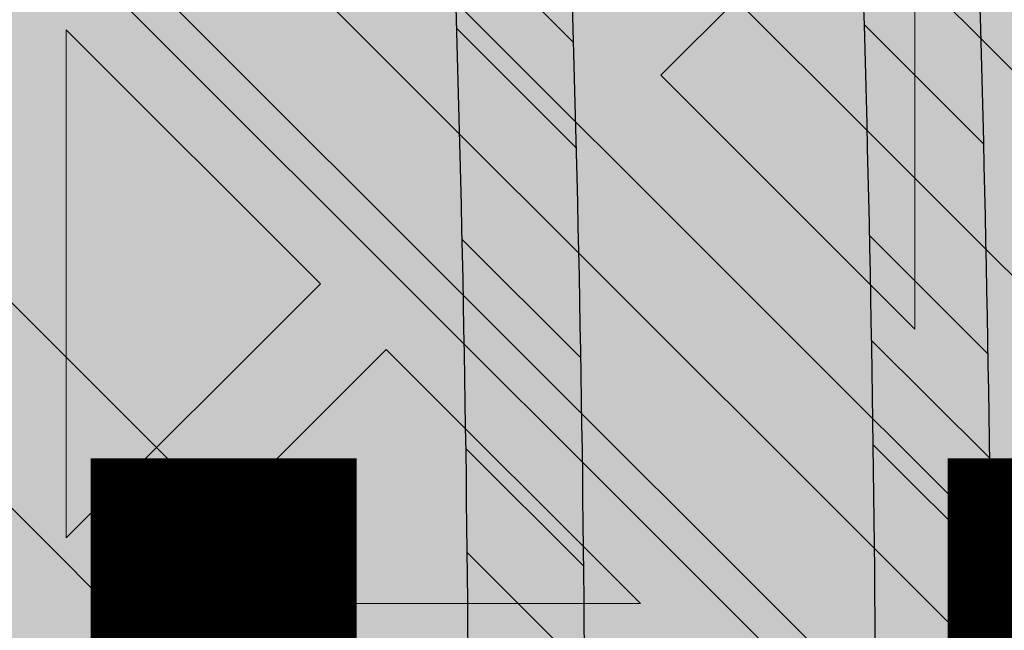
# Model space of a CAD drawing. Units: inches. Extents: x 844 to 2234, y 346 to 1084.
# Tile 80 of 93: x 2003.858 to 2006.557, y 703.938 to 705.614. Entities that reach past the tile are written whole.
import ezdxf

# ---------------------------------------------------------------- set-up
doc = ezdxf.new("R2010")
doc.units = ezdxf.units.IN
doc.header["$MEASUREMENT"] = 0
for name, color, linetype, lineweight in [('A-ANNO-DIMS', 2, 'Continuous', 18), ('furniture', 8, 'Continuous', 18), ('RA-AP-01$0$INT', 35, 'Continuous', 5)]:
    doc.layers.add(name, color=color, linetype=linetype, lineweight=lineweight)
doc.layers.add('RA-AP-01$0$FURN', color=3, linetype='Continuous')
doc.layers.add('RA-AP-01$0$WOOD', color=64, linetype='Continuous')
doc.styles.get("Standard").update_dxf_attribs({"font": 'arial.ttf'})
doc.dimstyles.get("Standard").update_dxf_attribs({"dimtxt": 6, "dimasz": 3, "dimexe": 0.18, "dimexo": 0.0625, "dimgap": 0.09, "dimtad": 0, "dimtih": 1, "dimtoh": 1, "dimdec": 1, "dimzin": 0, "dimdsep": 46, "dimlunit": 3, "dimtxsty": 'Standard', "dimblk": 'ARCHTICK', "dimcen": 0.09, "dimadec": 0, "dimazin": 0, "dimtfac": 1, "dimtdec": 1, "dimtofl": 0, "dimtmove": 0, "dimatfit": 3, "dimfxl": 1, "dimtolj": 1, "dimtzin": 0, "dimarcsym": 0})

# ---------------------------------------------------------------- blocks, each defined once
blk = doc.blocks.new('A$C18D01794')
at = {"layer": 'RA-AP-01$0$INT'}
h = blk.add_hatch(color=256, dxfattribs=at)
h.paths.add_polyline_path([(4.585917135068448, -7.856712009587804), (4.614201406330596, -7.856712009587056), (4.668846067270487, -7.802067348644738), (4.723490728212344, -7.856712009584164), (4.771774999457151, -7.856712009582887), (4.826419660396886, -7.80206734864072), (4.862780050090322, -7.838427738332541), (4.844495778842715, -7.856712009580965), (4.862780050090411, -7.856712009580482), (4.905206456960182, -7.814285602707865), (4.947632863832445, -7.856712009578238), (4.965917135079675, -7.856712009577755), (4.947632863831759, -7.838427738330656), (4.983993253523576, -7.802067348637219), (5.038637914464627, -7.856712009575829), (5.08692218571208, -7.856712009574554), (5.141566846649976, -7.802067348634224), (5.196211507589851, -7.856712009571666), (5.224495778822615, -7.856712009570916), (4.905206456953975, -7.537422687702283)])
h.paths.add_polyline_path([(4.895206456956031, -7.575706958950402), (4.895206456958921, -7.684996280828174), (4.840561796018589, -7.630351619890275)], flags=16)
h.paths.add_polyline_path([(4.915206456955638, -7.575706958949956), (4.969851117895509, -7.630351619887399), (4.915206456957609, -7.684996280827732)], flags=16)
h.paths.add_polyline_path([(4.826419660395175, -7.644493755514321), (4.881064321335613, -7.699138416452331), (4.771774999456703, -7.69913841645522)], flags=16)
h.paths.add_polyline_path([(4.983993253519558, -7.644493755510815), (5.038637914460456, -7.699138416449285), (4.929348592581548, -7.69913841645126)], flags=16)
h.paths.add_polyline_path([(4.881064321336025, -7.719138416452334), (4.826419660397532, -7.773783077393256), (4.771774999457062, -7.719138416455217)], flags=16)
h.paths.add_polyline_path([(4.929348592582019, -7.71913841645126), (5.038637914460982, -7.719138416449284), (4.983993253522945, -7.773783077389749)], flags=16)
h.paths.add_polyline_path([(4.895206456960191, -7.733280552075633), (4.895206456962115, -7.806001331460164), (4.876922185715016, -7.824285602708492), (4.840561796021581, -7.787925213016675)], flags=16)
h.paths.add_polyline_path([(4.915206456958487, -7.733280552075187), (4.969851117899527, -7.787925213013798), (4.933490728206909, -7.824285602708034), (4.9152064569598, -7.806001331461736)], flags=16)
h.paths.add_polyline_path([(4.757632863832376, -7.733280552079264), (4.812277524772842, -7.787925213017304), (4.757632863834348, -7.842569873958233)], flags=16)
h.paths.add_polyline_path([(4.737632863832376, -7.73328055207979), (4.737632863834348, -7.842569873958701), (4.682988202893906, -7.787925213020692)], flags=16)
h.paths.add_polyline_path([(5.05278005008503, -7.733280552072701), (5.052780050087917, -7.842569873951664), (4.998135389146995, -7.787925213013169)], flags=16)
h.paths.add_polyline_path([(5.072780050085024, -7.733280552072333), (5.127424711025931, -7.787925213010806), (5.072780050087916, -7.842569873951244)], flags=16)
h.paths.add_polyline_path([(4.935917135072783, -7.506712009583784), (5.255206456948811, -7.826001331459767), (5.255206456948932, -7.797717060211899), (5.200561796010279, -7.743072399273238), (5.255206456949403, -7.688427738334128), (5.25520645694961, -7.640143467086677), (5.200561796009787, -7.585498806146837), (5.236922185702417, -7.549138416454212), (5.255206456949919, -7.56742268770172), (5.255206456949998, -7.549138416454178), (5.212780050078687, -7.506712009583814), (5.25520645695036, -7.464285602712145), (5.255206456950438, -7.446001331464763), (5.236922185702424, -7.464285602712779), (5.200561796009796, -7.427925213020149), (5.255206456950753, -7.373280552079203), (5.25520645695096, -7.324996280834394), (5.200561796010322, -7.270351619893748), (5.255206456951428, -7.215706958952649), (5.255206456951547, -7.187422687705071)])
h.paths.add_polyline_path([(5.042988202883395, -7.42792521302065), (5.097632863823085, -7.373280552080975), (5.097632863822622, -7.482569873959883)], flags=16)
h.paths.add_polyline_path([(5.028846067259663, -7.442067348644384), (5.083490728198774, -7.496712009583504), (4.974201406321001, -7.496712009583035)], flags=16)
h.paths.add_polyline_path([(5.117632863823087, -7.37328055208089), (5.172277524762331, -7.42792521302015), (5.11763286382262, -7.482569873959851)], flags=16)
h.paths.add_polyline_path([(5.08349072819877, -7.516712009582191), (5.028846067259652, -7.571356670521302), (4.974201406320998, -7.516712009582638)], flags=16)
h.paths.add_polyline_path([(5.131774999446817, -7.35913841645716), (5.186419660386065, -7.413783077396415), (5.241064321325782, -7.359138416456712)], flags=17)
h.paths.add_polyline_path([(5.131774999446228, -7.496712009583703), (5.186419660386065, -7.442067348643883), (5.222780050079488, -7.478427738337313), (5.204495778832781, -7.496712009584014)], flags=16)
h.paths.add_polyline_path([(5.097632863822613, -7.530854145205813), (5.097632863823061, -7.640143467084723), (5.042988202883383, -7.585498806145032)], flags=16)
h.paths.add_polyline_path([(5.131774999446899, -7.339138416457162), (5.241064321325809, -7.339138416456712), (5.186419660386591, -7.284493755517479)], flags=17)
h.paths.add_polyline_path([(5.131774999446226, -7.516712009581999), (5.204495778830767, -7.516712009581702), (5.22278005007868, -7.534996280829206), (5.186419660386049, -7.571356670521828)], flags=16)
h.paths.add_polyline_path([(5.11763286382262, -7.530854145205852), (5.17227752476232, -7.585498806145562), (5.117632863823064, -7.64014346708481)], flags=16)
h.paths.add_polyline_path([(5.186419660386069, -7.599640941770585), (5.241064321325754, -7.654285602710281), (5.131774999446791, -7.654285602709814)], flags=16)
h.paths.add_polyline_path([(5.131774999446872, -7.674285602709813), (5.24106432132578, -7.674285602710282), (5.186419660386554, -7.728930263649504)], flags=16)
h.paths.add_polyline_path([(5.255206456951811, -7.126001331467467), (5.255206456951895, -7.106712009588038), (4.555206456956052, -7.106712009588038), (4.555206456956136, -7.12600133146746), (4.905206456953973, -7.476001331465289)])
h.paths.add_polyline_path([(4.983993253513404, -7.368930263651977), (4.92934859257295, -7.314285602713969), (5.03863791445186, -7.314285602711063)], flags=16)
h.paths.add_polyline_path([(4.969851117889988, -7.383072399276016), (4.915206456952556, -7.437717060215906), (4.915206456949648, -7.328427738338133)], flags=16)
h.paths.add_polyline_path([(4.929348592572535, -7.294285602713971), (4.983993253511019, -7.239640941773039), (5.038637914451496, -7.294285602711065)], flags=16)
h.paths.add_polyline_path([(5.052780050074912, -7.280143467087016), (4.998135389134438, -7.225498806148989), (5.052780050072919, -7.170854145208052)], flags=16)
h.paths.add_polyline_path([(5.07278005007491, -7.280143467086489), (5.072780050072918, -7.170854145207579), (5.127424711013374, -7.225498806145578)], flags=16)
h.paths.add_polyline_path([(4.89520645695295, -7.437717060216355), (4.840561796013067, -7.383072399278919), (4.895206456950961, -7.328427738338582)], flags=16)
h.paths.add_polyline_path([(4.915206456948365, -7.280143467090674), (4.915206456946434, -7.207422687704125), (4.933490728192729, -7.18913841645701), (4.969851117886972, -7.225498806149623)], flags=16)
h.paths.add_polyline_path([(4.881064321327021, -7.314285602715054), (4.82641966038902, -7.368930263655506), (4.771774999448108, -7.314285602717047)], flags=16)
h.paths.add_polyline_path([(4.895206456950073, -7.280143467091125), (4.840561796009022, -7.225498806152518), (4.876922185700835, -7.18913841645908), (4.895206456948749, -7.207422687706589)], flags=16)
h.paths.add_polyline_path([(4.983993253510392, -7.211356670525576), (4.947632863816944, -7.174996280833758), (4.965917135064043, -7.156712009585847), (5.038637914448995, -7.156712009584522)], flags=16)
h.paths.add_polyline_path([(4.881064321326543, -7.294285602715056), (4.771774999447578, -7.294285602717046), (4.826419660385607, -7.239640941776569)], flags=16)
h.paths.add_polyline_path([(4.905206456946447, -7.19913841645844), (4.862780050074785, -7.156712009587725), (4.947632863816685, -7.156712009586302)], flags=16)
h.paths.add_polyline_path([(5.14156684663679, -7.211356670521528), (5.086922185696452, -7.156712009583639), (5.196211507574223, -7.156712009581651)], flags=16)
h.paths.add_polyline_path([(4.8264196603837, -7.211356670529104), (4.771774999442643, -7.156712009590501), (4.8444957788276, -7.156712009588568), (4.862780050075511, -7.17499628083566)], flags=16)
h.paths.add_polyline_path([(4.812277524760289, -7.225498806153156), (4.757632863822258, -7.28014346709363), (4.757632863819352, -7.170854145214669)], flags=16)
h.paths.add_polyline_path([(4.73763286382226, -7.280143467093997), (4.682988202881349, -7.22549880615554), (4.737632863819352, -7.170854145215086)], flags=16)
h.paths.add_polyline_path([(4.723490728195188, -7.156712009591787), (4.668846067257299, -7.211356670532127), (4.614201406317417, -7.156712009594693)], flags=16)
h.paths.add_polyline_path([(4.597632863829262, -7.506712009583814), (4.555206456957951, -7.54913841645418), (4.555206456958029, -7.56742268770172), (4.573490728205535, -7.549138416454212), (4.609851117898167, -7.585498806146839), (4.555206456958338, -7.640143467086675), (4.555206456958546, -7.688427738334125), (4.60985111789767, -7.743072399273238), (4.555206456959015, -7.797717060211899), (4.555206456959138, -7.826001331459767), (4.874495778835167, -7.506712009583786), (4.5552064569564, -7.187422687705062), (4.555206456956523, -7.215706958952644), (4.609851117897629, -7.270351619893746), (4.555206456956988, -7.324996280834396), (4.555206456957198, -7.373280552079195), (4.609851117898153, -7.427925213020147), (4.573490728205528, -7.464285602712779), (4.555206456957507, -7.446001331464756), (4.555206456957585, -7.464285602712143)])
h.paths.add_polyline_path([(4.712780050085332, -7.482569873959882), (4.712780050084863, -7.373280552080972), (4.767424711024555, -7.42792521302065)], flags=16)
h.paths.add_polyline_path([(4.726922185709173, -7.496712009583504), (4.781566846648288, -7.442067348644384), (4.836211507586949, -7.496712009583033)], flags=16)
h.paths.add_polyline_path([(4.692780050085327, -7.482569873959851), (4.638135389145619, -7.427925213020149), (4.692780050084865, -7.373280552080892)], flags=16)
h.paths.add_polyline_path([(4.726922185709182, -7.516712009582191), (4.836211507586949, -7.51671200958264), (4.7815668466483, -7.571356670521304)], flags=16)
h.paths.add_polyline_path([(4.678637914461726, -7.496712009583706), (4.605917135075169, -7.496712009584014), (4.587632863828464, -7.478427738337311), (4.623993253521887, -7.442067348643881)], flags=16)
h.paths.add_polyline_path([(4.712780050085336, -7.530854145205816), (4.767424711024568, -7.585498806145034), (4.71278005008489, -7.640143467084724)], flags=16)
h.paths.add_polyline_path([(4.678637914461726, -7.516712009582001), (4.623993253521899, -7.571356670521829), (4.587632863829271, -7.534996280829206), (4.605917135077185, -7.5167120095817)], flags=16)
h.paths.add_polyline_path([(4.692780050085336, -7.530854145205848), (4.692780050084889, -7.64014346708481), (4.638135389145632, -7.585498806145562)], flags=16)
h.paths.add_polyline_path([(4.623993253521885, -7.413783077396415), (4.678637914461131, -7.359138416457161), (4.56934859258217, -7.359138416456712)], flags=17)
h.paths.add_polyline_path([(4.623993253521901, -7.599640941770568), (4.678637914461158, -7.654285602709814), (4.569348592582195, -7.654285602710281)], flags=16)
h.paths.add_polyline_path([(4.678637914461051, -7.339138416457162), (4.623993253521361, -7.284493755517479), (4.569348592582143, -7.339138416456712)], flags=17)
h.paths.add_polyline_path([(4.678637914461076, -7.674285602709813), (4.623993253521399, -7.728930263649504), (4.569348592582167, -7.674285602710281)], flags=16)
h = blk.add_hatch(color=256, dxfattribs=at)
h.paths.add_polyline_path([(4.905206456954232, -7.537422687702028), (4.874495778835232, -7.506712009583718), (4.555206456959138, -7.826001331459766), (4.555206456959269, -7.856712009588616), (4.585917135068449, -7.856712009587804)])
h.paths.add_polyline_path([(4.935917135072152, -7.506712009583152), (4.905206456953497, -7.537422687701806), (5.224495778822614, -7.856712009570917), (5.255206456948681, -7.856712009570104), (5.255206456948813, -7.826001331459768)])
h.paths.add_polyline_path([(5.255206456951549, -7.18742268770507), (5.255206456951813, -7.126001331467461), (4.905206456953563, -7.476001331465701), (4.935917135072559, -7.506712009584006)])
h.paths.add_polyline_path([(4.874495778835167, -7.506712009583785), (4.905206456953818, -7.476001331465132), (4.555206456956135, -7.126001331467458), (4.555206456956399, -7.187422687705064)])
h = blk.add_hatch(color=256, dxfattribs=at)
h.paths.add_polyline_path([(4.89520645695096, -7.328427738338579), (4.840561796013068, -7.383072399278921), (4.89520645695295, -7.437717060216353)])
h.paths.add_polyline_path([(4.915206456952557, -7.437717060215907), (4.969851117889986, -7.383072399276024), (4.915206456949648, -7.328427738338133)])
h.paths.add_polyline_path([(4.929348592572952, -7.31428560271397), (4.983993253513403, -7.368930263651974), (5.038637914451863, -7.314285602711064)])
h.paths.add_polyline_path([(5.038637914451498, -7.294285602711065), (4.983993253511018, -7.239640941773039), (4.929348592572535, -7.294285602713969)])
h.paths.add_polyline_path([(4.969851117886971, -7.225498806149624), (4.93349072819273, -7.189138416457011), (4.915206456946433, -7.207422687704124), (4.915206456948367, -7.280143467090678)])
h.paths.add_polyline_path([(4.965917135064045, -7.156712009585847), (4.947632863816945, -7.17499628083376), (4.983993253510389, -7.211356670525573), (5.038637914448995, -7.156712009584522)])
h.paths.add_polyline_path([(4.998135389134439, -7.22549880614899), (5.05278005007491, -7.280143467087016), (5.052780050072921, -7.170854145208054)])
h.paths.add_polyline_path([(5.072780050074911, -7.28014346708649), (5.127424711013374, -7.225498806145579), (5.072780050072921, -7.170854145207581)])
h.paths.add_polyline_path([(5.196211507574225, -7.156712009581651), (5.08692218569645, -7.156712009583639), (5.141566846636789, -7.211356670521529)])
h.paths.add_polyline_path([(4.862780050074782, -7.156712009587723), (4.90520645694645, -7.199138416458444), (4.94763286381669, -7.156712009586302)])
h.paths.add_polyline_path([(4.895206456950073, -7.280143467091126), (4.895206456948746, -7.207422687706587), (4.876922185700836, -7.189138416459078), (4.840561796009025, -7.225498806152521)])
h.paths.add_polyline_path([(4.826419660385605, -7.239640941776569), (4.771774999447577, -7.294285602717049), (4.881064321326541, -7.294285602715055)])
h.paths.add_polyline_path([(4.771774999448108, -7.314285602717046), (4.82641966038902, -7.368930263655505), (4.88106432132702, -7.314285602715054)])
h.paths.add_polyline_path([(4.757632863822258, -7.280143467093631), (4.812277524760285, -7.225498806153153), (4.757632863819352, -7.170854145214668)])
h.paths.add_polyline_path([(4.862780050075512, -7.17499628083566), (4.844495778827599, -7.156712009588567), (4.771774999442647, -7.156712009590504), (4.8264196603837, -7.211356670529104)])
h.paths.add_polyline_path([(4.682988202881349, -7.225498806155537), (4.737632863822258, -7.280143467093997), (4.737632863819352, -7.170854145215087)])
h.paths.add_polyline_path([(4.723490728195189, -7.156712009591783), (4.614201406317418, -7.156712009594692), (4.668846067257298, -7.211356670532127)])
h = blk.add_hatch(color=256, dxfattribs=at)
h.paths.add_polyline_path([(4.781566846647504, -7.442067348645805), (4.836211507586161, -7.496712009584463), (4.726922185708388, -7.496712009584918)])
h.paths.add_polyline_path([(4.836211507586161, -7.516712009584068), (4.781566846647504, -7.571356670522723), (4.726922185708388, -7.516712009583606)])
h.paths.add_polyline_path([(4.76742471102377, -7.585498806146453), (4.712780050084083, -7.640143467086137), (4.712780050084542, -7.530854145207227)])
h.paths.add_polyline_path([(4.692780050084544, -7.530854145207257), (4.692780050084084, -7.64014346708622), (4.638135389144834, -7.585498806146965)])
h.paths.add_polyline_path([(4.678637914460932, -7.516712009583407), (4.623993253521102, -7.571356670523233), (4.587632863827676, -7.53499628082981), (4.605917135074382, -7.516712009583104)])
h.paths.add_polyline_path([(4.573490728204743, -7.54913841645434), (4.60985111789737, -7.585498806146969), (4.555206456957541, -7.640143467086797), (4.555206456957237, -7.567422687701846)])
h.paths.add_polyline_path([(4.623993253521098, -7.599640941770699), (4.67863791446035, -7.654285602709951), (4.56934859258139, -7.654285602710407)])
h.paths.add_polyline_path([(4.678637914460275, -7.67428560270995), (4.623993253520583, -7.728930263649637), (4.56934859258136, -7.674285602710405)])
h.paths.add_polyline_path([(4.609851117896854, -7.743072399273369), (4.555206456958196, -7.797717060212026), (4.555206456957738, -7.688427738334254)])
h.paths.add_polyline_path([(4.597632863828475, -7.506712009583301), (4.555206456957283, -7.549138416454495), (4.555206456956805, -7.464285602712587)])
h.paths.add_polyline_path([(4.678637914460932, -7.496712009585113), (4.605917135076396, -7.496712009585417), (4.587632863828479, -7.478427738337913), (4.623993253521104, -7.442067348645284)])
h.paths.add_polyline_path([(4.692780050084091, -7.373280552082301), (4.692780050084548, -7.482569873961267), (4.638135389144834, -7.427925213021552)])
h.paths.add_polyline_path([(4.767424711023772, -7.427925213022072), (4.712780050084545, -7.48256987396129), (4.712780050084089, -7.373280552082384)])
h.paths.add_polyline_path([(4.67863791446036, -7.359138416457298), (4.623993253521105, -7.41378307739655), (4.569348592581399, -7.35913841645684)])
h.paths.add_polyline_path([(4.609851117897371, -7.427925213020278), (4.573490728204743, -7.464285602712907), (4.555206456957237, -7.446001331465401), (4.555206456957548, -7.373280552080448)])
h.paths.add_polyline_path([(4.623993253520596, -7.284493755517612), (4.67863791446028, -7.339138416457299), (4.569348592581367, -7.339138416456838)])
h.paths.add_polyline_path([(4.609851117896867, -7.270351619893878), (4.555206456957749, -7.324996280832994), (4.55520645695821, -7.21570695895522)])
for p, q in [((4.905206456953975, -7.476001331465289), (4.555206456956136, -7.12600133146746)), ((4.874495778835167, -7.506712009583786), (4.555206456956399, -7.187422687705064)), ((4.771774999448109, -7.314285602717045), (4.881064321327019, -7.314285602715054)), ((4.826419660389018, -7.368930263655503), (4.771774999448109, -7.314285602717045)), ((4.881064321327019, -7.314285602715054), (4.82641966038902, -7.368930263655505)), ((4.895206456950956, -7.328427738338584), (4.840561796013068, -7.383072399278921)), ((4.895206456950959, -7.328427738338582), (4.89520645695295, -7.437717060216353)), ((4.767424711024554, -7.42792521302065), (4.712780050084865, -7.373280552080972)), ((4.712780050084865, -7.373280552080972), (4.71278005008533, -7.482569873959882)), ((4.89520645695295, -7.437717060216353), (4.840561796013068, -7.383072399278921)), ((4.71278005008533, -7.482569873959882), (4.767424711024555, -7.427925213020651))]:
    blk.add_line(p, q, dxfattribs=at)
blk = doc.blocks.new('A$C32926AE1')
at = {"layer": 'RA-AP-01$0$FURN'}
h = blk.add_hatch(dxfattribs=at)
h.set_pattern_fill('ANSI31', color=256, scale=0.1, style=0)
h.set_pattern_definition([(45, (0, 0), (-0.0088388347648318, 0.0088388347648318), [])])
edge = h.paths.add_edge_path(flags=16)
edge.add_arc((4.904771284329206, 4.246793130718756), 0.2603971832811541, 75.22398030683196, 104.7760196931204)
edge.add_arc((4.904771284329206, 4.246793130718756), 0.2603971832811541, 75.223980306832, 104.77601969312039, ccw=False)
edge = h.paths.add_edge_path(flags=16)
edge.add_arc((4.904771284329206, 4.067062675376612), 0.2603971832811541, 255.2239803068796, 284.776019693168)
edge.add_arc((4.904771284329206, 4.067062675376612), 0.2603971832811541, 255.22398030687958, 284.77601969316805, ccw=False)
edge = h.paths.add_edge_path(flags=0)
edge.add_arc((4.904771284329206, 4.067062675376612), 0.2603971832811541, 255.2239803068796, 284.776019693168)
edge.add_arc((4.904771284329206, 4.067062675376612), 0.2603971832811541, 255.22398030687958, 284.77601969316805, ccw=False)
edge = h.paths.add_edge_path(flags=0)
edge.add_arc((4.904771284329206, 4.067062675376612), 0.2603971832811541, 255.2239803068796, 284.776019693168)
edge.add_arc((4.904771284329206, 4.067062675376612), 0.2603971832811541, 255.22398030687958, 284.77601969316805, ccw=False)
edge = h.paths.add_edge_path()
edge.add_arc((4.604388392048174, 4.588829985554312), 0.1599999999999918, 342.3781640246255, 354.4317409793762)
edge.add_arc((5.090145208887507, 4.43216705527679), 0.3503971832811637, 162.0091218307731, 180.3186872093483)
edge.add_arc((5.205154176610243, 4.588829985554953), 0.1599999999999917, 185.5682590208461, 197.6218359767349)
edge.add_arc((4.904771284329229, 4.246793130718735), 0.3503971832811761, 72.00912183053516, 107.9908781690354)
edge.add_arc((9.535952835716557, 4.28682295566602), 4.798342501046485, 178.2875002453811, 181.5576802719453)
edge.add_arc((4.719397359771122, 4.43216705527679), 0.3503971832811637, 359.6813127906516, 377.9908781692269)
edge.add_arc((9.535967292294904, 4.286822350292874), 4.778371420254705, 178.2965938931842, 181.5667745797229)
edge.add_arc((4.719397359771122, 4.43216705527679), 0.3303971832811637, 359.6813127906516, 377.9908781692269)
edge.add_arc((0.2735752763637294, 4.286822350292874), 4.7783714202547, 358.4332254202771, 361.7034061068158)
edge.add_arc((5.061434214606998, 4.732549947558029), 0.1600000000000254, 252.3781640250584, 264.4317409792362)
edge.add_arc((4.748108354051257, 4.732549947558012), 0.1600000000000541, 275.5682590208426, 287.6218359759532)
edge.add_arc((4.604388392048115, 4.588829985554317), 0.1800000000000505, 342.3567572500182, 349.3735009646207)
edge.add_arc((5.205154176610254, 4.588829985554976), 0.1800000000000069, 190.6264990356027, 197.6432427513933)
edge.add_arc((5.061434214607106, 4.732549947558013), 0.1800000000000424, 252.3567572496606, 259.3735009644582)
edge.add_arc((4.904771284329208, 4.246793130718737), 0.3303971832811676, 71.99844483668534, 108.0015551637021)
edge.add_arc((4.748108354051414, 4.732549947558045), 0.1800000000000547, 280.6264990355479, 287.6432427495938)
edge.add_arc((5.090145208887514, 4.432167055276789), 0.2803971832811691, 162.8706300666893, 180.816523289902)
edge.add_arc((4.719397359771136, 4.432167055276689), 0.2803971832811534, 359.183476710103, 377.1293699333214)
edge.add_arc((4.904771284329222, 4.246793130718737), 0.2803971832811769, 72.87063006672916, 107.1293699332334)
edge.add_arc((5.090145208887522, 4.432167055276788), 0.2603971832811776, 165.2239803068007, 180.9953123810312)
edge.add_arc((4.719397359771141, 4.432167055276699), 0.2603971832811458, 359.0046876189768, 374.7760196932087)
edge.add_arc((5.090145208887507, 4.43216705527679), 0.3303971832811637, 162.0091218307731, 180.3186872093483)
edge.add_arc((9.53595427642584, 4.285015535491528), 4.728345371032053, 178.265043920078, 181.5679956281801)
edge.add_arc((0.2735882922327999, 4.285015535491582), 4.728345371032045, 358.4320043718193, 361.7349560799204)
edge.add_arc((9.535953591267507, 4.284458026472751), 4.708343996644348, 178.2573054306777, 181.5704995759608)
edge.add_arc((0.273588977391114, 4.284458026472785), 4.708343996644358, 358.4295004240388, 361.7426945693213)
edge.add_arc((0.2735889773911131, 4.029397779622582), 4.708343996644359, 358.2573054306787, 361.5704995759613)
edge.add_arc((9.535953591267518, 4.029397779622618), 4.708343996644359, 178.4295004240391, 181.7426945693223)
edge.add_arc((0.2735882922327901, 4.028840270603786), 4.728345371032054, 358.2650439200796, 361.5679956281808)
edge.add_arc((9.53595427642584, 4.028840270603841), 4.728345371032054, 178.4320043718199, 181.7349560799219)
edge.add_arc((0.2735752763637302, 4.027033455802493), 4.778371420254699, 358.2965938931842, 361.5667745797229)
edge.add_arc((4.719397359771122, 3.881688750818578), 0.3303971832811637, 342.0091218307731, 360.3186872093484)
edge.add_arc((5.090145208887507, 3.881688750818578), 0.3303971832811637, 179.6813127906516, 197.9908781692269)
edge.add_arc((9.535967292294904, 4.027033455802493), 4.778371420254705, 178.433225420277, 181.7034061068158)
edge.add_arc((4.719397359771122, 3.881688750818578), 0.3503971832811637, 342.0091218307731, 360.3186872093484)
edge.add_arc((9.53595283571655, 4.027032850429349), 4.79834250104648, 178.4423197280546, 181.7124997546188)
edge.add_arc((4.719397359771141, 3.881688750818669), 0.2603971832811458, 345.2239803067913, 360.9953123810232)
edge.add_arc((5.090145208887522, 3.88168875081858), 0.2603971832811776, 179.0046876189687, 194.7760196931993)
edge.add_arc((4.904771284329222, 4.067062675376631), 0.2803971832811769, 252.8706300667665, 287.1293699332708)
edge.add_arc((4.719397359771136, 3.881688750818678), 0.2803971832811534, 342.8706300666787, 360.8165232898969)
edge.add_arc((5.090145208887514, 3.881688750818579), 0.2803971832811691, 179.183476710098, 197.1293699333106)
edge.add_arc((4.748108354051414, 3.581305858537323), 0.1800000000000547, 72.3567572504062, 79.37350096445199)
edge.add_arc((4.904771284329208, 4.067062675376631), 0.3303971832811676, 251.9984448362979, 288.0015551633146)
edge.add_arc((5.061434214607106, 3.581305858537355), 0.1800000000000424, 100.6264990355418, 107.6432427503394)
edge.add_arc((5.205154176610254, 3.725025820540392), 0.1800000000000069, 162.3567572486066, 169.3735009643972)
edge.add_arc((4.604388392048115, 3.725025820541051), 0.1800000000000505, 10.62649903537925, 17.64324274998182)
edge.add_arc((4.748108354051257, 3.581305858537356), 0.1600000000000541, 72.37816402404681, 84.43174097915735)
edge.add_arc((4.904771284329229, 4.067062675376632), 0.3503971832811761, 252.0091218309645, 287.9908781694648)
edge.add_arc((5.061434214606998, 3.581305858537339), 0.1600000000000254, 95.56825902076373, 107.6218359749416)
edge.add_arc((5.205154176610243, 3.725025820540414), 0.1599999999999917, 162.3781640232651, 174.4317409791539)
edge.add_arc((5.090145208887507, 3.881688750818578), 0.3503971832811637, 179.6813127906516, 197.9908781692269)
edge.add_arc((4.604388392048174, 3.725025820541056), 0.1599999999999918, 5.568259020623824, 17.62183597537444)
edge.add_arc((0.2735897329420762, 4.28682295566602), 4.798342501046482, 358.4423197280547, 361.7124997546188)
edge.add_arc((0.2735897329420691, 4.027032850429348), 4.798342501046489, 358.2875002453812, 361.5576802719453)
at = {"layer": 'RA-AP-01$0$WOOD'}
h = blk.add_hatch(color=256, dxfattribs=at)
h.dxf.hatch_style = 1
h.paths.add_polyline_path([(5.157430609644524, 4.573483066760929, -0.1009492694046607), (5.155401577623758, 4.593365984175333, -0.1842662638101597), (5.172249623284174, 4.638795604568598, 0.2056608120311276), (5.179560981299304, 4.661316324430096, 0.3614336704623542), (5.134352340494423, 4.706524965234944, 0.2056608120311297), (5.111831620632933, 4.699213607219793, -0.1842662638101113), (5.066402000239693, 4.682365561559342, -0.1055311479399994), (5.045656153913092, 4.68467289944697, 0.1567636581983829), (4.763886414745334, 4.684672899446966, -0.1055311479399895), (4.743140568418733, 4.68236556155934, -0.1842662638100833), (4.6977109480255, 4.69921360721979, 0.2056608120302612), (4.675190228164109, 4.706524965234949, 0.3614336704708441), (4.629981587358889, 4.66131632442871, 0.2056608120245944), (4.637292945374126, 4.638795604567974, -0.1842662638101024), (4.654140991034615, 4.59336598417475, -0.1009492694055169), (4.652111959013835, 4.573483066760181, 0.021410119221476), (4.629748025606143, 4.156712009541676, 0.0214101192214795), (4.652111959013809, 3.739940952323101, -0.1009492694059586), (4.654140991034615, 3.720058034908448, -0.1842662638100975), (4.637292945374126, 3.674628414515226, 0.2056608120245705), (4.629981587358889, 3.652107694654492, 0.3614336704708879), (4.675190228164113, 3.606899053848249, 0.2056608120302384), (4.697710948025501, 3.614210411863408, -0.1842662638100995), (4.743140568418738, 3.63105845752386, -0.1055311479402541), (4.763886414745388, 3.628751119636215, 0.1567636581983776), (5.045656153913137, 3.628751119636244, -0.1055311479397538), (5.066402000239692, 3.631058457523857, -0.1842662638101067), (5.111831620632931, 3.614210411863407, 0.2056608120310924), (5.134352340494417, 3.606899053848256, 0.3614336704624001), (5.179560981299307, 3.652107694653103, 0.2056608120311314), (5.172249623284175, 3.6746284145146, -0.1842662638101402), (5.155401577623758, 3.72005803490786, -0.1009492694051366), (5.15743060964455, 3.739940952322354, 0.0214101192215073), (5.179794543052287, 4.156712009541468, 0.0214101192215252)])
h.paths.add_polyline_path([(4.639748609479751, 4.156712009541513, 0.0213537860821624), (4.661970494867118, 3.741887061152232, -0.094075836301374), (4.664143710413708, 3.7196126951003, -0.1824818158568985), (4.644813765429836, 3.668037719127816, 0.2056608120245319), (4.639939526753007, 3.653023905887301, 0.3614336704710246), (4.676106439397173, 3.616856993242342, 0.2056608120302234), (4.691120252638095, 3.621731231919122, -0.1824818158602558), (4.742695228611606, 3.641061176902986, -0.1029891339458722), (4.766991894714349, 3.638256818950944, 0.156709409989566), (5.042550673941472, 3.638256818950105, -0.102989133958497), (5.066847340047078, 3.641061176902949, -0.1824818158594995), (5.118422316020358, 3.621731231919103, 0.2056608120311416), (5.133436129261316, 3.616856993242346, 0.3614336704621468), (5.169603041905217, 3.653023905886178, 0.2056608120310986), (5.164728803228477, 3.668037719127177, -0.1824818158565612), (5.145398858244737, 3.719612695099578, -0.0940758363009313), (5.147572073791232, 3.741887061151398, 0.0213537860822023), (5.169793959178681, 4.156712009541451, 0.0213537860822226), (5.147572073791203, 4.571536957931898, -0.0940758363005034), (5.145398858244737, 4.59381132398362, -0.1824818158565587), (5.164728803228476, 4.645386299956021, 0.2056608120311045), (5.169603041905216, 4.66040011319702, 0.3614336704621845), (5.133436129261313, 4.696567025840856, 0.2056608120310773), (5.118422316020359, 4.691692787164098, -0.182481815859508), (5.066847340047078, 4.67236284218025, -0.1029891339584606), (5.04255067394148, 4.675167200133092, 0.156709409989566), (4.766991894714357, 4.675167200132257, -0.1029891339458842), (4.742695228611611, 4.672362842180213, -0.1824818158602725), (4.691120252638095, 4.691692787164077, 0.2056608120302152), (4.676106439397174, 4.696567025840858, 0.3614336704710363), (4.639939526753005, 4.660400113195899, 0.2056608120245495), (4.644813765429837, 4.645386299955384, -0.1824818158568934), (4.664143710413708, 4.593811323982902, -0.0940758363009187), (4.661970494867149, 4.571536957931074, 0.021353786082177)], flags=16)
h.paths.add_polyline_path([(5.129794543052235, 4.432167055276933, -0.0141661062790638), (5.130152669293814, 4.156927903047693, -0.0141661062790647), (5.129794543052234, 3.881688750818433, -0.0785247771143638), (5.10979738006795, 3.755143611847103, 0.0945969212073497), (5.105408519571111, 3.717898134952927, 0.1043170707844957), (5.116074640131521, 3.670385395016088, 0.1043170707864965), (5.068561900193738, 3.681051515576561, 0.09459692119553), (5.031316423304057, 3.676662655080835, -0.1580239521427272), (4.778226145355827, 3.676662655080367, 0.0945969211986668), (4.740980668464973, 3.681051515576592, 0.1043170707882822), (4.693467928526415, 3.670385395015844, 0.1043170707867916), (4.704134049087309, 3.717898134953662, 0.0945969211972894), (4.69974518859162, 3.755143611844042, -0.0785247771163196), (4.679748025606343, 3.881688750818406, -0.0141661062790663), (4.679389899364763, 4.156927903047693, -0.0141661062790672), (4.679748025606343, 4.432167055276998, -0.0785247771163064), (4.699745188591625, 4.55871219425134, 0.094596921197333), (4.704134049087308, 4.595957671141738, 0.1043170707867205), (4.693467928526416, 4.643470411079523, 0.1043170707882628), (4.740980668464965, 4.632804290518776, 0.0945969211988114), (4.778226145355874, 4.637193151015016, -0.158023952142669), (5.031316423304015, 4.637193151014546, 0.0945969211956361), (5.068561900193736, 4.632804290518806, 0.1043170707864979), (5.11607464013152, 4.643470411079278, 0.1043170707844617), (5.105408519571112, 4.595957671142455, 0.0945969212074597), (5.109797380067959, 4.558712194248236, -0.0785247771143467)], flags=0)
h.paths.add_polyline_path([(5.119794532311105, 4.432259799204851, -0.0142000800617244), (5.120156169157484, 4.156927903047701, -0.0142000800617277), (5.119794532311105, 3.881596006890482, -0.0784894509520253), (5.100273383573699, 3.758192358677797, 0.0940138827242913), (5.095413455884425, 3.717477693979438, 0.0606271852308753), (5.099615656341024, 3.686844378806616, 0.0606271852322524), (5.068982341167493, 3.691046579263239, 0.0940138827010453), (5.028267676478798, 3.686186651576848, -0.1580706864508061), (4.781274892180912, 3.686186651576435, 0.0940138827026903), (4.740560227491556, 3.691046579263279, 0.0606271852339895), (4.709926912317155, 3.686844378806508, 0.0606271852329405), (4.714129112773991, 3.717477693980356, 0.094013882701304), (4.709269185087677, 3.758192358669163, -0.0784894509577193), (4.689748036347473, 3.881596006890469, -0.014200080061729), (4.689386399501094, 4.156927903047709, -0.0142000800617217), (4.689748036347473, 4.432259799204808, -0.078489450957724), (4.709269185087651, 4.555663447426125, 0.0940138827014585), (4.714129112773992, 4.596378112114996, 0.0606271852329731), (4.709926912317154, 4.62701142728886, 0.0606271852340196), (4.74056022749157, 4.622809226832087, 0.0940138827024997), (4.781274892180847, 4.627669154518912, -0.1580706864508359), (5.028267676478777, 4.627669154518526, 0.0940138827010946), (5.068982341167492, 4.622809226832129, 0.060627185232254), (5.099615656341024, 4.627011427288751, 0.0606271852308727), (5.095413455884425, 4.59637811211593, 0.0940138827241088), (5.100273383573675, 4.555663447417647, -0.0784894509520978)], flags=0)
h.paths.add_polyline_path([(5.06978912287499, 4.430218106756144, -0.014241683694547), (5.070173729147532, 4.156927903047672, -0.0142416836945458), (5.06978912287499, 3.883637699339223, -0.0800609523125196), (5.052662118612511, 3.773463122773442, 0.0526421978001116), (5.04590916754064, 3.740550867606997, 0.0526421977992423), (5.012996912374707, 3.73379791653534, -0.1583028414718258), (4.796545656286308, 3.73379791653451, 0.0526421978034211), (4.763633401117837, 3.740550867607021, 0.0526421978018622), (4.756880450045755, 3.773463122774558, -0.0800609523117106), (4.739753445783639, 3.883637699339268, -0.0142416836945435), (4.739368839511098, 4.156927903047671, -0.0142416836945477), (4.739753445783639, 4.430218106756155, -0.0800609523116345), (4.75688045004574, 4.540392683320762, 0.052642197801941), (4.763633401117837, 4.573304938488346, 0.0526421978035071), (4.796545656286361, 4.580057889560873, -0.1583028414717561), (5.012996912374669, 4.580057889560039, 0.0526421977993048), (5.04590916754064, 4.57330493848837, 0.0526421978002057), (5.052662118612529, 4.540392683321868, -0.080060952312477)], flags=0)
h.paths.add_polyline_path([(5.049789715110557, 4.43038092723357, -0.0143097550741839), (5.05018085590259, 4.156927903047715, -0.0143097550741854), (5.049789715110558, 3.883474878861827, -0.0800685599149176), (5.03362098255317, 3.779581877367999, 0.0306258898956367), (5.028241146483733, 3.758218888663947, 0.0306258898977031), (5.006878157778253, 3.75283905259408, -0.1583983521624096), (4.802664410878162, 3.752839052594731, 0.0306258898946014), (4.781301422174808, 3.758218888663924, 0.0306258898967912), (4.775921586105202, 3.779581877368794, -0.080068559914251), (4.759752853548071, 3.883474878861786, -0.0143097550741854), (4.759361712756037, 4.156927903047671, -0.0143097550741854), (4.759752853548071, 4.430380927233557, -0.0800685599142479), (4.775921586105193, 4.534273928726546, 0.0306258898968306), (4.781301422174808, 4.555636917431444, 0.0306258898945754), (4.802664410878143, 4.561016753500631, -0.1583983521624168), (5.006878157778244, 4.561016753501291, 0.0306258898977177), (5.028241146483733, 4.555636917431421, 0.0306258898958182), (5.03362098255321, 4.534273928727244, -0.080068559914796)], flags=0)
h.paths.add_polyline_path([(4.999766070382627, 4.428171244713864, -0.0143443147609634), (5.000198441819402, 4.156927903047689, -0.0143443147609612), (4.999766070382627, 3.885684561381556, -0.0784641635803329), (4.987356730658798, 3.799103304488872, -0.1506053783831347), (4.822185837999821, 3.79910330448882, -0.0784641635803318), (4.809776498276007, 3.885684561381509, -0.014344314760963), (4.809344126839227, 4.156927903047677, -0.0143443147609645), (4.809776498276007, 4.428171244713873, -0.0784641635803192), (4.822185837999822, 4.514752501606549, -0.1506053783831338), (4.987356730658798, 4.514752501606494, -0.078464163580285)], flags=0)
h.paths.add_polyline_path([(4.979755254238824, 4.42764379880488, -0.0143772539198268), (4.980205517789977, 4.156927903047693, -0.0143772539198275), (4.979755254238824, 3.886212007290489, -0.0689242507424422), (4.971183264704897, 3.815276770442801, -0.1296645318904179), (4.838359303953726, 3.815276770442746, -0.0689242507424186), (4.829787314419809, 3.886212007290419, -0.0143772539198292), (4.829337050868653, 4.156927903047653, -0.0143772539198325), (4.829787314419809, 4.427643798804946, -0.0689242507424211), (4.838359303953725, 4.498579035652621, -0.1296645318904187), (4.971183264704897, 4.498579035652565, -0.0689242507424401)], flags=0)
h = blk.add_hatch(color=256, dxfattribs=at)
h.dxf.hatch_style = 1
h.paths.add_polyline_path([(5.145398858244737, 4.59381132398362, -0.1824818158565616), (5.164728803228476, 4.645386299956021, 0.2056608120311045), (5.169603041905216, 4.66040011319702, 0.3614336704621845), (5.133436129261313, 4.696567025840856, 0.2056608120310773), (5.118422316020359, 4.691692787164098, -0.182481815859508), (5.066847340047078, 4.67236284218025, -0.1029891339584606), (5.04255067394148, 4.675167200133092, 0.156709409989566), (4.766991894714357, 4.675167200132257, -0.1029891339458842), (4.742695228611611, 4.672362842180213, -0.1824818158602725), (4.691120252638095, 4.691692787164077, 0.2056608120302152), (4.676106439397174, 4.696567025840858, 0.3614336704710363), (4.639939526753005, 4.660400113195899, 0.2056608120245495), (4.644813765429837, 4.645386299955384, -0.1824818158568934), (4.664143710413708, 4.593811323982902, -0.0940758363009187), (4.661970494867149, 4.571536957931074, 0.0213537860821772), (4.639748609479751, 4.156712009541507, 0.0213537860821625), (4.661970494867119, 3.741887061152226, -0.0940758363013071), (4.664143710413708, 3.719612695100309, -0.1824818158569294), (4.644813765429836, 3.668037719127816, 0.2056608120245319), (4.639939526753007, 3.653023905887301, 0.3614336704710246), (4.676106439397173, 3.616856993242342, 0.2056608120302234), (4.691120252638095, 3.621731231919122, -0.1824818158602558), (4.742695228611606, 3.641061176902986, -0.1029891339458722), (4.766991894714349, 3.638256818950944, 0.156709409989566), (5.042550673941472, 3.638256818950105, -0.102989133958497), (5.066847340047078, 3.641061176902949, -0.1824818158594995), (5.118422316020358, 3.621731231919103, 0.2056608120311416), (5.133436129261316, 3.616856993242346, 0.3614336704621468), (5.169603041905217, 3.653023905886178, 0.2056608120310986), (5.164728803228477, 3.668037719127177, -0.1824818158565612), (5.145398858244737, 3.719612695099578, -0.0940758363009313), (5.147572073791232, 3.741887061151398, 0.0213537860822023), (5.169793959178681, 4.156712009541451, 0.0213537860822226), (5.147572073791203, 4.571536957931898, -0.0940758363004996)])
h.paths.add_polyline_path([(5.109797380067958, 4.55871219424824, -0.0785247771143472), (5.129794543052234, 4.432167055276936, -0.0141661062790644), (5.130152669293814, 4.156927903047685, -0.014166106279066), (5.129794543052234, 3.881688750818401, -0.0785247771143517), (5.109797380067946, 3.755143611847092, 0.0945969212073132), (5.105408519571111, 3.717898134952929, 0.1043170707844995), (5.116074640131521, 3.670385395016088, 0.1043170707864965), (5.068561900193738, 3.681051515576561, 0.09459692119553), (5.031316423304057, 3.676662655080835, -0.1580239521427272), (4.778226145355827, 3.676662655080367, 0.0945969211986668), (4.740980668464973, 3.681051515576592, 0.1043170707882822), (4.693467928526415, 3.670385395015844, 0.1043170707867916), (4.704134049087309, 3.717898134953662, 0.0945969211972894), (4.69974518859162, 3.755143611844042, -0.0785247771163196), (4.679748025606343, 3.881688750818406, -0.0141661062790663), (4.679389899364763, 4.156927903047693, -0.0141661062790672), (4.679748025606343, 4.432167055276998, -0.0785247771163064), (4.699745188591625, 4.55871219425134, 0.094596921197333), (4.704134049087308, 4.595957671141738, 0.1043170707867205), (4.693467928526416, 4.643470411079523, 0.1043170707882628), (4.740980668464965, 4.632804290518776, 0.0945969211988114), (4.778226145355874, 4.637193151015016, -0.158023952142669), (5.031316423304015, 4.637193151014546, 0.0945969211956361), (5.068561900193736, 4.632804290518806, 0.1043170707864979), (5.11607464013152, 4.643470411079278, 0.1043170707844617), (5.105408519571112, 4.595957671142455, 0.0945969212074504)], flags=16)
h.paths.add_polyline_path([(5.100273383573655, 4.55566344741771, -0.0784894509521388), (5.119794532311105, 4.432259799204852, -0.0142000800617252), (5.120156169157484, 4.156927903047686, -0.014200080061726), (5.119794532311105, 3.881596006890502, -0.0784894509520446), (5.100273383573696, 3.758192358677786, 0.0940138827242721), (5.095413455884425, 3.717477693979436, 0.0606271852308692), (5.099615656341024, 3.686844378806616, 0.0606271852322522), (5.068982341167493, 3.691046579263239, 0.0940138827010453), (5.028267676478798, 3.686186651576848, -0.1580706864508061), (4.781274892180912, 3.686186651576435, 0.0940138827026903), (4.740560227491556, 3.691046579263279, 0.0606271852339895), (4.709926912317155, 3.686844378806508, 0.0606271852329405), (4.714129112773991, 3.717477693980356, 0.094013882701304), (4.709269185087677, 3.758192358669163, -0.0784894509577193), (4.689748036347473, 3.881596006890469, -0.014200080061729), (4.689386399501094, 4.156927903047709, -0.0142000800617217), (4.689748036347473, 4.432259799204808, -0.078489450957724), (4.709269185087651, 4.555663447426125, 0.0940138827014585), (4.714129112773992, 4.596378112114996, 0.0606271852329731), (4.709926912317154, 4.62701142728886, 0.0606271852340196), (4.74056022749157, 4.622809226832087, 0.0940138827024997), (4.781274892180847, 4.627669154518912, -0.1580706864508359), (5.028267676478777, 4.627669154518526, 0.0940138827010946), (5.068982341167492, 4.622809226832129, 0.060627185232254), (5.099615656341024, 4.627011427288751, 0.0606271852308727), (5.095413455884425, 4.59637811211593, 0.094013882723957)], flags=0)
h.paths.add_polyline_path([(5.04590916754064, 4.57330493848837, 0.0526421978002057), (5.052662118612529, 4.540392683321868, -0.0800609523124783), (5.06978912287499, 4.430218106756142, -0.0142416836945469), (5.070173729147532, 4.156927903047672, -0.0142416836945458), (5.06978912287499, 3.883637699339223, -0.0800609523125196), (5.052662118612511, 3.773463122773442, 0.0526421978001116), (5.04590916754064, 3.740550867606997, 0.0526421977992423), (5.012996912374707, 3.73379791653534, -0.1583028414718258), (4.796545656286308, 3.73379791653451, 0.0526421978034211), (4.763633401117837, 3.740550867607021, 0.0526421978018622), (4.756880450045755, 3.773463122774558, -0.0800609523117106), (4.739753445783639, 3.883637699339268, -0.0142416836945435), (4.739368839511098, 4.156927903047671, -0.0142416836945477), (4.739753445783639, 4.430218106756155, -0.0800609523116345), (4.75688045004574, 4.540392683320762, 0.052642197801941), (4.763633401117837, 4.573304938488346, 0.0526421978035071), (4.796545656286361, 4.580057889560873, -0.1583028414717561), (5.012996912374669, 4.580057889560039, 0.0526421977993048)], flags=0)
h.paths.add_polyline_path([(5.028241146483733, 4.555636917431422, 0.0306258898956949), (5.033620982553182, 4.534273928727329, -0.0800685599148649), (5.049789715110557, 4.430380927233569, -0.0143097550741839), (5.05018085590259, 4.156927903047715, -0.0143097550741854), (5.049789715110558, 3.883474878861827, -0.0800685599149176), (5.03362098255317, 3.779581877367999, 0.0306258898956367), (5.028241146483733, 3.758218888663947, 0.0306258898977031), (5.006878157778253, 3.75283905259408, -0.1583983521624096), (4.802664410878162, 3.752839052594731, 0.0306258898946014), (4.781301422174808, 3.758218888663924, 0.0306258898967912), (4.775921586105202, 3.779581877368794, -0.080068559914251), (4.759752853548071, 3.883474878861786, -0.0143097550741854), (4.759361712756037, 4.156927903047671, -0.0143097550741854), (4.759752853548071, 4.430380927233557, -0.0800685599142479), (4.775921586105193, 4.534273928726546, 0.0306258898968306), (4.781301422174808, 4.555636917431444, 0.0306258898945754), (4.802664410878143, 4.561016753500631, -0.1583983521624168), (5.006878157778244, 4.561016753501291, 0.0306258898977174)], flags=0)
h.paths.add_polyline_path([(4.987356730658798, 4.514752501606494, -0.0784641635803018), (4.999766070382627, 4.428171244713845, -0.0143443147609637), (5.000198441819402, 4.156927903047665, -0.0143443147609622), (4.999766070382628, 3.885684561381514, -0.0784641635802952), (4.987356730658797, 3.799103304488872, -0.1506053783831338), (4.822185837999821, 3.799103304488819, -0.0784641635803342), (4.809776498276007, 3.885684561381512, -0.0143443147609628), (4.809344126839227, 4.156927903047676, -0.0143443147609646), (4.809776498276007, 4.428171244713873, -0.0784641635803192), (4.822185837999822, 4.514752501606549, -0.1506053783831338)], flags=0)
h.paths.add_polyline_path([(4.971183264704897, 4.498579035652566, -0.0689242507424384), (4.979755254238824, 4.427643798804883, -0.0143772539198276), (4.980205517789977, 4.15692790304768, -0.0143772539198258), (4.979755254238823, 3.88621200729051, -0.0689242507424628), (4.971183264704897, 3.815276770442801, -0.129664531890417), (4.838359303953726, 3.815276770442746, -0.0689242507424186), (4.829787314419809, 3.886212007290419, -0.0143772539198292), (4.829337050868653, 4.156927903047653, -0.0143772539198325), (4.829787314419809, 4.427643798804946, -0.0689242507424211), (4.838359303953725, 4.498579035652621, -0.1296645318904187)], flags=0)
h = blk.add_hatch(dxfattribs=at)
h.set_pattern_fill('ANSI31', color=256, scale=0.05, style=0)
h.set_pattern_definition([(45, (0, 0), (-0.0044194173824159, 0.0044194173824159), [])])
h.paths.add_polyline_path([(5.130152669293814, 4.156927903047704, 0.0141661062790657), (5.129794543052234, 4.432167055276982, 0.0777827904001433), (5.110168979996553, 4.557559993161921, -0.0976515123401879), (5.105408519571111, 4.595957671142454, -0.1043170707844687), (5.116074640131522, 4.64347041107928), (5.099615656341024, 4.627011427288751, 0.0606271852308727), (5.095413455884425, 4.59637811211593, 0.0940138827241088), (5.100273383573675, 4.555663447417647, -0.0784894509520972), (5.119794532311105, 4.432259799204852, -0.0142000800617252), (5.120156169157484, 4.156927903047686, -0.014200080061726), (5.119794532311105, 3.881596006890502, -0.0784894509520446), (5.100273383573696, 3.758192358677786, 0.0940138827242721), (5.095413455884425, 3.717477693979436, 0.0606271852308692), (5.099615656341024, 3.686844378806616), (5.116074640131519, 3.67038539501609, -0.1043170707844594), (5.105408519571112, 3.717898134952912, -0.0976515123401594), (5.11016897999655, 3.756295812933435, 0.0777827904001654), (5.129794543052234, 3.881688750818409, 0.0141661062790665)])
h.paths.add_polyline_path([(5.030164222210597, 3.676291055149937, -0.0976515123472002), (5.068561900193739, 3.681051515576561, -0.1043170707864927), (5.116074640131521, 3.670385395016088), (5.099615656341024, 3.686844378806616, 0.0606271852322522), (5.068982341167493, 3.691046579263239, 0.0940138827010453), (5.028267676478798, 3.686186651576848, -0.1580706864508061), (4.781274892180912, 3.686186651576435, 0.0940138827026903), (4.740560227491556, 3.691046579263279, 0.0606271852339913), (4.709926912317154, 3.686844378806508), (4.693467928526416, 3.670385395015845, -0.1043170707882796), (4.740980668464973, 3.681051515576592, -0.0976515123427246), (4.779378346446416, 3.676291055150394, 0.156512506893803)])
h.paths.add_polyline_path([(4.689748036347473, 3.881596006890472, -0.014200080061729), (4.689386399501094, 4.156927903047712, -0.0142000800617195), (4.689748036347473, 4.432259799204768, -0.078489450957742), (4.709269185087648, 4.555663447426114, 0.0940138827014821), (4.714129112773992, 4.596378112114995, 0.0606271852329748), (4.709926912317154, 4.62701142728886), (4.693467928526414, 4.643470411079524, -0.1043170707867939), (4.704134049087309, 4.595957671141706, -0.09765151234893), (4.699373588660725, 4.557559993157876, 0.0777827903975372), (4.679748025606343, 4.432167055276987, 0.0141661062790675), (4.679389899364763, 4.156927903047675, 0.0141661062790641), (4.679748025606343, 3.88168875081843, 0.0777827903975637), (4.699373588660724, 3.756295812937497, -0.0976515123490278), (4.704134049087308, 3.717898134953629, -0.1043170707867196), (4.693467928526416, 3.670385395015845), (4.709926912317155, 3.686844378806508, 0.0606271852329413), (4.714129112773991, 3.717477693980357, 0.0940138827013084), (4.709269185087676, 3.758192358669166, -0.0784894509577192)])
h.paths.add_polyline_path([(4.779378346446434, 4.63756475094498, -0.0976515123427943), (4.740980668464964, 4.632804290518776, -0.1043170707882609), (4.693467928526416, 4.643470411079523), (4.709926912317154, 4.62701142728886, 0.0606271852340196), (4.74056022749157, 4.622809226832087, 0.0940138827024997), (4.781274892180847, 4.627669154518912, -0.1580706864508359), (5.028267676478777, 4.627669154518526, 0.0940138827010946), (5.068982341167492, 4.622809226832129, 0.060627185232254), (5.099615656341024, 4.627011427288751), (5.116074640131521, 4.643470411079279, -0.1043170707865022), (5.068561900193735, 4.632804290518806, -0.0976515123475899), (5.030164222210446, 4.637564750945479, 0.1565125068936924)])
h = blk.add_hatch(dxfattribs=at)
h.set_pattern_fill('ANSI32', color=256, scale=0.2, style=0)
h.set_pattern_definition([(45, (0, 0), (-0.0530330085889911, 0.0530330085889911), []), (45, (0.035355339, 0), (-0.0530330085889911, 0.0530330085889911), [])])
h.paths.add_polyline_path([(5.119794532311105, 4.432259799204823, 0.0777015974868765), (5.10065834347252, 4.554469821747928, -0.0968902511992216), (5.095413455884425, 4.596378112115931, -0.060627185230871), (5.099615656341024, 4.627011427288751, -0.060627185232254), (5.068982341167492, 4.622809226832129, -0.0968902512198245), (5.027074050790956, 4.628054114423209, 0.1564657949319105), (4.782468517866163, 4.628054114422785, -0.0968902512152247), (4.740560227491555, 4.622809226832088, -0.0606271852339878), (4.709926912317155, 4.627011427288859, -0.0606271852329413), (4.714129112773991, 4.596378112115011, -0.0968902512205338), (4.708884225182929, 4.554469821738175, 0.0777015974804443), (4.689748036347473, 4.43225979920482, 0.0142000800617215), (4.689386399501094, 4.156927903047726, 0.0142000800617273), (4.689748036347473, 3.88159600689052, 0.077701597480541), (4.708884225182985, 3.759385984357019, -0.096890251220082), (4.714129112773992, 3.717477693980371, -0.0606271852329731), (4.709926912317154, 3.686844378806507, -0.060627185233988), (4.740560227491554, 3.691046579263279, -0.0968902512152569), (4.782468517866175, 3.685801691672578, 0.1564657949319236), (5.027074050790988, 3.685801691672169, -0.0968902512197451), (5.068982341167491, 3.691046579263239, -0.0606271852322557), (5.099615656341024, 3.686844378806616, -0.0606271852308727), (5.095413455884425, 3.717477693979438, -0.0968902511991229), (5.100658343472507, 3.7593859843474, 0.0777015974868745), (5.119794532311105, 3.8815960068905, 0.014200080061726), (5.120156169157484, 4.156927903047685, 0.0142000800617238)])
h.paths.add_polyline_path([(5.070173729147531, 4.156927903047684, -0.0142416836945481), (5.06978912287499, 3.883637699339191, -0.0800609523125107), (5.052662118612505, 3.773463122773424, 0.0526421978000811), (5.04590916754064, 3.740550867606997, 0.0526421977993214), (5.012996912374658, 3.733797916535325, -0.1583028414717916), (4.796545656286304, 3.733797916534512, 0.0526421978034138), (4.763633401117837, 3.740550867607021, 0.0526421978018622), (4.756880450045755, 3.773463122774558, -0.0800609523117106), (4.739753445783639, 3.883637699339268, -0.0142416836945435), (4.739368839511098, 4.156927903047671, -0.0142416836945477), (4.739753445783639, 4.430218106756155, -0.0800609523116345), (4.75688045004574, 4.540392683320762, 0.052642197801941), (4.763633401117837, 4.573304938488346, 0.0526421978035071), (4.796545656286361, 4.580057889560873, -0.1583028414717561), (5.012996912374669, 4.580057889560039, 0.0526421977993048), (5.04590916754064, 4.57330493848837, 0.0526421978002057), (5.052662118612529, 4.540392683321868, -0.0800609523124783), (5.06978912287499, 4.430218106756142, -0.0142416836945463)], flags=16)
h.paths.add_polyline_path([(5.050180855902591, 4.156927903047686, -0.0143097550741856), (5.049789715110558, 3.883474878861795, -0.0800685599148126), (5.033620982553202, 3.7795818773681, 0.0306258898957837), (5.028241146483733, 3.758218888663947, 0.0306258898977031), (5.006878157778253, 3.75283905259408, -0.1583983521624096), (4.802664410878162, 3.752839052594731, 0.0306258898946014), (4.781301422174808, 3.758218888663924, 0.0306258898967912), (4.775921586105202, 3.779581877368794, -0.080068559914251), (4.759752853548071, 3.883474878861786, -0.0143097550741854), (4.759361712756037, 4.156927903047671, -0.0143097550741854), (4.759752853548071, 4.430380927233557, -0.0800685599142479), (4.775921586105193, 4.534273928726546, 0.0306258898968306), (4.781301422174808, 4.555636917431444, 0.0306258898945754), (4.802664410878143, 4.561016753500631, -0.1583983521624168), (5.006878157778244, 4.561016753501291, 0.0306258898977177), (5.028241146483733, 4.555636917431421, 0.0306258898958182), (5.03362098255321, 4.534273928727244, -0.0800685599147973), (5.049789715110557, 4.430380927233568, -0.0143097550741854)], flags=0)
h.paths.add_polyline_path([(5.000198441819402, 4.15692790304769, -0.0143443147609622), (4.999766070382627, 3.885684561381539, -0.0784641635803169), (4.987356730658798, 3.799103304488873, -0.1506053783831347), (4.822185837999821, 3.79910330448882, -0.0784641635803318), (4.809776498276007, 3.885684561381509, -0.014344314760963), (4.809344126839227, 4.156927903047677, -0.0143443147609645), (4.809776498276007, 4.428171244713873, -0.0784641635803192), (4.822185837999822, 4.514752501606549, -0.1506053783831338), (4.987356730658798, 4.514752501606494, -0.0784641635803018), (4.999766070382627, 4.428171244713845, -0.0143443147609624)], flags=0)
h.paths.add_polyline_path([(4.980205517789976, 4.156927903047707, -0.0143772539198295), (4.979755254238824, 3.886212007290466, -0.06892425074242), (4.971183264704897, 3.815276770442801, -0.129664531890417), (4.838359303953726, 3.815276770442746, -0.0689242507424186), (4.829787314419809, 3.886212007290419, -0.0143772539198292), (4.829337050868653, 4.156927903047653, -0.0143772539198325), (4.829787314419809, 4.427643798804946, -0.0689242507424211), (4.838359303953725, 4.498579035652621, -0.1296645318904187), (4.971183264704897, 4.498579035652565, -0.0689242507424418), (4.979755254238824, 4.427643798804878, -0.0143772539198259)], flags=0)
for centre, radius, start, end in [((9.535952835716557, 4.28682295566602), 4.798342501046485, 178.2875002453811, 181.5576802719453), ((9.535967292294904, 4.286822350292874), 4.778371420254705, 178.2965938931842, 181.5667745797229), ((9.53595427642584, 4.285015535491528), 4.728345371032053, 178.265043920078, 181.5679956281801), ((9.535953591267507, 4.284458026472751), 4.708343996644348, 178.2573054306777, 181.5704995759608)]:
    blk.add_arc(centre, radius, start, end, dxfattribs=at)
blk = doc.blocks.new('A$C5D2F253E')
at = {"layer": 'RA-AP-01$0$FURN', "xscale": -0.7999999999883585, "yscale": 0.7999999999883585, "zscale": 0.8, "rotation": 90}
blk.add_blockref('A$C18D01794', (-5.687757199772477, 4.75791982714071), dxfattribs=at)
at = {"layer": 'RA-AP-01$0$WOOD', "rotation": 270}
blk.add_blockref('A$C32926AE1', (-4.161339601644158, 5.73852594588169), dxfattribs=at)
blk = doc.blocks.new('_ArchTick')
at = {"color": 0, "linetype": 'ByBlock', "const_width": 0.15}
blk.add_lwpolyline([(-0.5, -0.5), (0.5, 0.5)], dxfattribs=at)
blk = doc.blocks.new('*D121')
at = {"layer": 'A-ANNO-DIMS', "color": 0, "lineweight": -2, "transparency": 16777216}
for p, q in [((2030.271987351997, 734.262611118704), (2040.245275089302, 734.262611118704)), ((2040.065275089302, 734.262611118704), (2040.065275089302, 704.6043509484256)), ((2040.065275089302, 668.557359536674), (2040.065275089302, 698.2156197069523)), ((2030.271987351997, 668.557359536674), (2040.245275089302, 668.557359536674))]:
    blk.add_line(p, q, dxfattribs=at)
at = {"layer": 'Defpoints', "color": 0, "transparency": 16777216}
for p in [(2030.209487351997, 734.262611118704), (2040.065275089302, 734.262611118704), (2030.209487351997, 668.557359536674)]:
    blk.add_point(p, dxfattribs=at)
at = {"layer": 'A-ANNO-DIMS', "color": 0, "lineweight": -2, "transparency": 16777216, "xscale": 3, "yscale": 3, "zscale": 3}
for p, rotation in [((2040.065275089302, 734.262611118704), 90), ((2040.065275089302, 668.557359536674), 270)]:
    blk.add_blockref('_ArchTick', p, dxfattribs=dict(at, rotation=rotation))
at = {"layer": 'A-ANNO-DIMS', "color": 0, "transparency": 16777216, "insert": (2040.065275089302, 701.4099853276883), "char_height": 6, "attachment_point": 5}
blk.add_mtext('\\A1;LOUNGE SET 5\'-5 1/2" TYP.', dxfattribs=at)

msp = doc.modelspace()

# ---------------------------------------------------------------- block references
at = {"layer": 'furniture', "xscale": -15.94108302203742, "yscale": 15.94108302203742, "zscale": 15.94108302203742, "rotation": 270}
msp.add_blockref('A$C5D2F253E', (1990.567271852805, 701.4028671565849), dxfattribs=at)

# ---------------------------------------------------------------- dimensions: what is measured, and where the dimension line sits
at = {"layer": 'A-ANNO-DIMS'}
dim = msp.add_linear_dim(base=(2040.065275089302, 734.262611118704), p1=(2030.209487351996, 668.5573595366737), p2=(2030.209487351996, 734.2626111187037), angle=90, text='LOUNGE SET <> TYP.', dimstyle='Standard', override={"dimdec": 1, "dimlfac": 1, "dimrnd": 0, "dimzin": 1, "dimdsep": 46, "dimlunit": 4, "dimfrac": 2}, dxfattribs=at)
dim.commit()
dim.dimension.update_dxf_attribs({"geometry": '*D121', "text_midpoint": (2040.065275089302, 701.4099853276883)})

doc.saveas('drawing.dxf')
